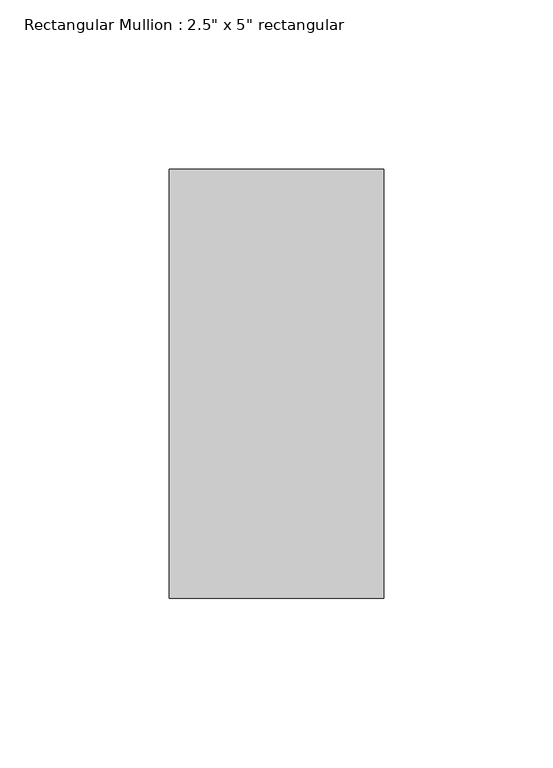
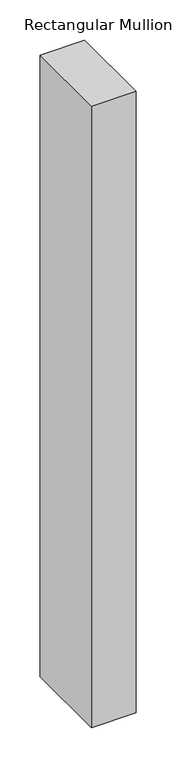
"""IFC4 building model written with IfcOpenShell, lengths in millimetres: member geometry."""

from ifc_helpers import new_model, si_unit, frame, origin, place, context, project, spatial, polyline, outline, extrude, source, transform, mapped, element, save


def member_e557a406(model_context):
    return source(origin(), model_context, "Body", "SweptSolid", [
        extrude(outline(polyline([(0.0, 63.5), (0.0, -63.5), (-63.5, -63.5), (-63.5, 63.5), (0.0, 63.5)])), frame((0.0, 0.0, -939.8), z_axis=(0.0, 0.0, 1.0), x_axis=(1.0, 0.0, 0.0)), (0.0, 0.0, 1.0), 939.8),
    ])


if __name__ == "__main__":
    model = new_model("IFC4")
    model_context = context("Model", 3, world=origin())
    ifc_project = project(units=[si_unit("LENGTHUNIT", "METRE", prefix="MILLI")], contexts=[model_context])
    site = spatial("IfcSite", under=ifc_project)
    building = spatial("IfcBuilding", under=site)
    placement = place(None, origin())
    member_shape = member_e557a406(model_context)
    element("IfcMember", 1, ObjectType="Rectangular Mullion : 2.5\" x 5\" rectangular", at=placement, inside=building, context=model_context, shape_type="MappedRepresentation", body=[
        mapped(member_shape, transform((0.0, 0.0, 0.0), x_axis=(1.0, 0.0, 0.0), y_axis=(0.0, 1.0, 0.0), z_axis=(0.0, 0.0, 1.0))),
    ])
    save(model, "model.ifc")

# Revit data of these elements
# Type "Rectangular Mullion : 2.5\" x 5\" rectangular"
#   built-in parameter 1007304 = 0.416667 (stored number, unit not read)
#   built-in parameter 1007301 = 0.104167 (stored number, unit not read)
#   built-in parameter 1007300 = 0.104167 (stored number, unit not read)
# Element 1 (IfcMember, "Rectangular Mullion : 2.5\" x 5\" rectangular")
#   Materials on its faces: "Aluminum"
# Materials
#   "Aluminum": class "Metal", colour RGB 247 247 247, transparency 0, Description = "Aluminum 6061", Cost = 0
